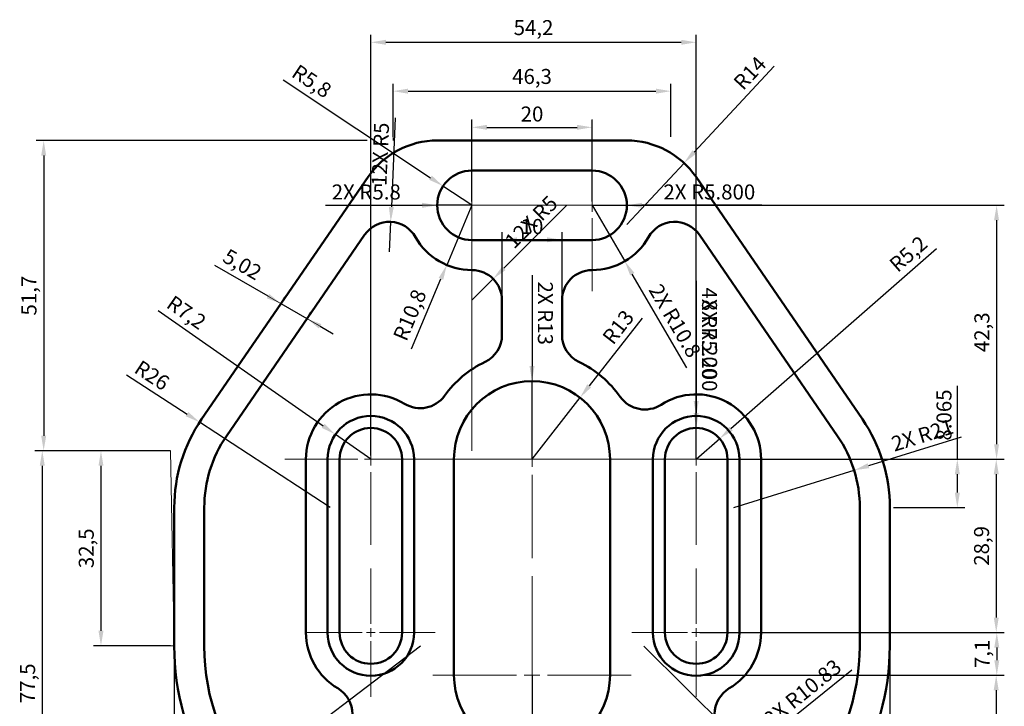
# Model space of a CAD drawing. Units: millimetres. Extents: x 11989 to 12153, y 10398 to 10572.
# Tile 2 of 2: x 11989 to 12153, y 10458 to 10572. Entities that reach past the tile are written whole.
import ezdxf

# ---------------------------------------------------------------- set-up
doc = ezdxf.new("R2010")
doc.units = ezdxf.units.MM
doc.linetypes.add('CENTER', pattern=[50.8, 31.75, -6.35, 6.35, -6.35])
for name, color, linetype, lineweight in [('M-CNTR', 1, 'CENTER', 18), ('M-CONS', 8, 'Continuous', 13), ('M-DIMS', 2, 'Continuous', 25), ('M-OUTL', 7, 'Continuous', 50)]:
    doc.layers.add(name, color=color, linetype=linetype, lineweight=lineweight)
doc.styles.get("Standard").update_dxf_attribs({"font": 'arial.ttf'})
doc.dimstyles.new('ISO-25', dxfattribs={"dimtxt": 2.5, "dimasz": 2.5, "dimexe": 1.25, "dimexo": 0.625, "dimtad": 1, "dimtxsty": 'Standard', "dimcen": 2.5, "dimadec": 0, "dimazin": 0, "dimtfac": 1, "dimtmove": 0, "dimatfit": 3, "dimfxl": 1, "dimarcsym": 0})

# ---------------------------------------------------------------- blocks, each defined once
blk = doc.blocks.new('*U5')
at = {"layer": 'M-CNTR', "color": 0, "transparency": 16777216}
for p, q in [((0, 1.44), (0, 10.7)), ((-10.7, 0), (-1.44, 0)), ((1.44, 0), (10.7, 0)), ((0, -10.7), (0, -1.44))]:
    blk.add_line(p, q, dxfattribs=at)
at = {"layer": 'M-CNTR', "color": 0, "linetype": 'Continuous', "transparency": 16777216}
for p, q in [((-0.72, 0), (0.72, 0)), ((0, -0.72), (0, 0.72))]:
    blk.add_line(p, q, dxfattribs=at)
blk = doc.blocks.new('*U6')
at = {"layer": 'M-CNTR', "color": 0, "transparency": 16777216}
for p, q in [((0, 1.44), (0, 10.7)), ((-10.7, 0), (-1.44, 0)), ((1.44, 0), (10.7, 0)), ((0, -10.7), (0, -1.44))]:
    blk.add_line(p, q, dxfattribs=at)
at = {"layer": 'M-CNTR', "color": 0, "linetype": 'Continuous', "transparency": 16777216}
for p, q in [((-0.72, 0), (0.72, 0)), ((0, -0.72), (0, 0.72))]:
    blk.add_line(p, q, dxfattribs=at)
blk = doc.blocks.new('*U7')
at = {"layer": 'M-CNTR', "color": 0, "transparency": 16777216}
for p, q in [((0, 2.16), (0, 14.3)), ((-14.3, 0), (-2.16, 0)), ((2.16, 0), (14.3, 0)), ((0, -14.3), (0, -2.16))]:
    blk.add_line(p, q, dxfattribs=at)
at = {"layer": 'M-CNTR', "color": 0, "linetype": 'Continuous', "transparency": 16777216}
for p, q in [((-1.08, 0), (1.08, 0)), ((0, -1.08), (0, 1.08))]:
    blk.add_line(p, q, dxfattribs=at)
blk = doc.blocks.new('*U8')
at = {"layer": 'M-CNTR', "color": 0, "transparency": 16777216}
for p, q in [((0, 2.16), (0, 14.3)), ((-14.3, 0), (-2.16, 0)), ((2.16, 0), (14.3, 0)), ((0, -14.3), (0, -2.16))]:
    blk.add_line(p, q, dxfattribs=at)
at = {"layer": 'M-CNTR', "color": 0, "linetype": 'Continuous', "transparency": 16777216}
for p, q in [((-1.08, 0), (1.08, 0)), ((0, -1.08), (0, 1.08))]:
    blk.add_line(p, q, dxfattribs=at)
blk = doc.blocks.new('*U9')
at = {"layer": 'M-CNTR', "color": 0, "transparency": 16777216}
for p, q in [((0, 2.16), (0, 14.3)), ((-14.3, 0), (-2.16, 0)), ((2.16, 0), (14.3, 0)), ((0, -14.3), (0, -2.16))]:
    blk.add_line(p, q, dxfattribs=at)
at = {"layer": 'M-CNTR', "color": 0, "linetype": 'Continuous', "transparency": 16777216}
for p, q in [((-1.08, 0), (1.08, 0)), ((0, -1.08), (0, 1.08))]:
    blk.add_line(p, q, dxfattribs=at)
blk = doc.blocks.new('*U10')
at = {"layer": 'M-CNTR', "color": 0, "transparency": 16777216}
for p, q in [((0, 2.16), (0, 14.3)), ((-14.3, 0), (-2.16, 0)), ((2.16, 0), (14.3, 0)), ((0, -14.3), (0, -2.16))]:
    blk.add_line(p, q, dxfattribs=at)
at = {"layer": 'M-CNTR', "color": 0, "linetype": 'Continuous', "transparency": 16777216}
for p, q in [((-1.08, 0), (1.08, 0)), ((0, -1.08), (0, 1.08))]:
    blk.add_line(p, q, dxfattribs=at)
blk = doc.blocks.new('*U11')
at = {"layer": 'M-CNTR', "color": 0, "transparency": 16777216}
for p, q in [((0, 2.6), (0, 16.5)), ((-16.5, 0), (-2.6, 0)), ((2.6, 0), (16.5, 0)), ((0, -16.5), (0, -2.6))]:
    blk.add_line(p, q, dxfattribs=at)
at = {"layer": 'M-CNTR', "color": 0, "linetype": 'Continuous', "transparency": 16777216}
for p, q in [((-1.3, 0), (1.3, 0)), ((0, -1.3), (0, 1.3))]:
    blk.add_line(p, q, dxfattribs=at)
blk = doc.blocks.new('*U12')
at = {"layer": 'M-CNTR', "color": 0, "transparency": 16777216}
for p, q in [((0, 2.6), (0, 16.5)), ((-16.5, 0), (-2.6, 0)), ((2.6, 0), (16.5, 0)), ((0, -16.5), (0, -2.6))]:
    blk.add_line(p, q, dxfattribs=at)
at = {"layer": 'M-CNTR', "color": 0, "linetype": 'Continuous', "transparency": 16777216}
for p, q in [((-1.3, 0), (1.3, 0)), ((0, -1.3), (0, 1.3))]:
    blk.add_line(p, q, dxfattribs=at)
blk = doc.blocks.new('*D15')
at = {"layer": 'Defpoints', "color": 0, "transparency": 16777216}
for p in [(12014.43, 10479.37), (12133.63, 10479.37), (12133.63, 10399.46)]:
    blk.add_point(p, dxfattribs=at)
at = {"layer": 'M-DIMS', "color": 0, "lineweight": -2, "transparency": 16777216}
for p, q in [((12014.43, 10478.74), (12014.43, 10398.21)), ((12133.63, 10478.74), (12133.63, 10398.21)), ((12016.93, 10399.46), (12131.13, 10399.46))]:
    blk.add_line(p, q, dxfattribs=at)
at = {"layer": 'M-DIMS', "color": 0, "transparency": 16777216}
for points in [[(12016.93, 10399.88), (12016.93, 10399.04), (12014.43, 10399.46)], [(12131.13, 10399.88), (12131.13, 10399.04), (12133.63, 10399.46)]]:
    blk.add_solid(points, dxfattribs=at)
at = {"layer": 'M-DIMS', "color": 0, "transparency": 16777216, "insert": (12074.03, 10401.59), "char_height": 2.5, "attachment_point": 5}
blk.add_mtext('119,2', dxfattribs=at)
blk = doc.blocks.new('*D16')
at = {"layer": 'Defpoints', "color": 0, "transparency": 16777216}
for p in [(12014.43, 10500.37), (12002.23, 10467.87), (12014.43, 10467.87)]:
    blk.add_point(p, dxfattribs=at)
at = {"layer": 'M-DIMS', "color": 0, "lineweight": -2, "transparency": 16777216}
for p, q in [((12013.8, 10500.37), (12000.98, 10500.37)), ((12002.23, 10497.87), (12002.23, 10470.37)), ((12013.8, 10467.87), (12000.98, 10467.87))]:
    blk.add_line(p, q, dxfattribs=at)
at = {"layer": 'M-DIMS', "color": 0, "transparency": 16777216}
for points in [[(12001.81, 10497.87), (12002.64, 10497.87), (12002.23, 10500.37)], [(12001.81, 10470.37), (12002.64, 10470.37), (12002.23, 10467.87)]]:
    blk.add_solid(points, dxfattribs=at)
at = {"layer": 'M-DIMS', "color": 0, "transparency": 16777216, "insert": (12000.1, 10484.12), "char_height": 2.5, "attachment_point": 5, "rotation": 90}
blk.add_mtext('32,5', dxfattribs=at)
blk = doc.blocks.new('*D17')
at = {"layer": 'Defpoints', "color": 0, "transparency": 16777216}
for p in [(12084.03, 10554.26), (12064.03, 10541.27), (12084.03, 10541.27)]:
    blk.add_point(p, dxfattribs=at)
at = {"layer": 'M-DIMS', "color": 0, "lineweight": -2, "transparency": 16777216}
for p, q in [((12064.03, 10541.9), (12064.03, 10555.51)), ((12084.03, 10541.9), (12084.03, 10555.51)), ((12066.53, 10554.26), (12081.53, 10554.26))]:
    blk.add_line(p, q, dxfattribs=at)
at = {"layer": 'M-DIMS', "color": 0, "transparency": 16777216}
for points in [[(12066.53, 10554.68), (12066.53, 10553.85), (12064.03, 10554.26)], [(12081.53, 10554.68), (12081.53, 10553.85), (12084.03, 10554.26)]]:
    blk.add_solid(points, dxfattribs=at)
at = {"layer": 'M-DIMS', "color": 0, "transparency": 16777216, "insert": (12074.03, 10556.16), "char_height": 2.5, "attachment_point": 5}
blk.add_mtext('20', dxfattribs=at)
blk = doc.blocks.new('*D18')
at = {"layer": 'Defpoints', "color": 0, "transparency": 16777216}
for p in [(12097.18, 10560.29), (12050.88, 10552.07), (12097.18, 10552.07)]:
    blk.add_point(p, dxfattribs=at)
at = {"layer": 'M-DIMS', "color": 0, "lineweight": -2, "transparency": 16777216}
for p, q in [((12050.88, 10552.7), (12050.88, 10561.54)), ((12097.18, 10552.7), (12097.18, 10561.54)), ((12053.38, 10560.29), (12094.68, 10560.29))]:
    blk.add_line(p, q, dxfattribs=at)
at = {"layer": 'M-DIMS', "color": 0, "transparency": 16777216}
for points in [[(12053.38, 10560.71), (12053.38, 10559.87), (12050.88, 10560.29)], [(12094.68, 10560.71), (12094.68, 10559.87), (12097.18, 10560.29)]]:
    blk.add_solid(points, dxfattribs=at)
at = {"layer": 'M-DIMS', "color": 0, "transparency": 16777216, "insert": (12074.03, 10562.42), "char_height": 2.5, "attachment_point": 5}
blk.add_mtext('46,3', dxfattribs=at)
blk = doc.blocks.new('*D19')
at = {"layer": 'Defpoints', "color": 0, "transparency": 16777216}
for p in [(12101.38, 10568.43), (12047.18, 10498.97), (12101.38, 10498.97)]:
    blk.add_point(p, dxfattribs=at)
at = {"layer": 'M-DIMS', "color": 0, "lineweight": -2, "transparency": 16777216}
for p, q in [((12047.18, 10499.6), (12047.18, 10569.68)), ((12101.38, 10499.6), (12101.38, 10569.68)), ((12049.68, 10568.43), (12098.88, 10568.43))]:
    blk.add_line(p, q, dxfattribs=at)
at = {"layer": 'M-DIMS', "color": 0, "transparency": 16777216}
for points in [[(12049.68, 10568.85), (12049.68, 10568.02), (12047.18, 10568.43)], [(12098.88, 10568.85), (12098.88, 10568.02), (12101.38, 10568.43)]]:
    blk.add_solid(points, dxfattribs=at)
at = {"layer": 'M-DIMS', "color": 0, "transparency": 16777216, "insert": (12074.28, 10570.56), "char_height": 2.5, "attachment_point": 5}
blk.add_mtext('54,2', dxfattribs=at)
blk = doc.blocks.new('*D20')
at = {"layer": 'Defpoints', "color": 0, "transparency": 16777216}
for p in [(12099.35, 10548.32), (12089.81, 10538.07)]:
    blk.add_point(p, dxfattribs=at)
at = {"layer": 'M-DIMS', "color": 0, "lineweight": -2, "transparency": 16777216}
for p, q in [((12114.38, 10564.45), (12101.06, 10550.15)), ((12089.81, 10538.07), (12099.35, 10548.32))]:
    blk.add_line(p, q, dxfattribs=at)
at = {"layer": 'M-DIMS', "color": 0, "transparency": 16777216}
blk.add_solid([(12100.75, 10550.43), (12101.36, 10549.86), (12099.35, 10548.32)], dxfattribs=at)
at = {"layer": 'M-DIMS', "color": 0, "transparency": 16777216, "insert": (12110.55, 10563.09), "char_height": 2.5, "attachment_point": 5, "rotation": 47.0295}
blk.add_mtext('R14', dxfattribs=at)
blk = doc.blocks.new('*D21')
at = {"layer": 'Defpoints', "color": 0, "transparency": 16777216}
for p in [(12059.2, 10544.48), (12064.03, 10541.27)]:
    blk.add_point(p, dxfattribs=at)
at = {"layer": 'M-DIMS', "color": 0, "lineweight": -2, "transparency": 16777216}
for p, q in [((12032.57, 10562.19), (12057.12, 10545.87)), ((12064.03, 10541.27), (12059.2, 10544.48))]:
    blk.add_line(p, q, dxfattribs=at)
at = {"layer": 'M-DIMS', "color": 0, "transparency": 16777216}
blk.add_solid([(12057.35, 10546.21), (12056.89, 10545.52), (12059.2, 10544.48)], dxfattribs=at)
at = {"layer": 'M-DIMS', "color": 0, "transparency": 16777216, "insert": (12037.16, 10561.69), "char_height": 2.5, "attachment_point": 5, "rotation": 326.3843}
blk.add_mtext('R5,8', dxfattribs=at)
blk = doc.blocks.new('*D22')
at = {"layer": 'Defpoints', "color": 0, "transparency": 16777216}
for p in [(12041.28, 10503.1), (12047.18, 10498.97)]:
    blk.add_point(p, dxfattribs=at)
at = {"layer": 'M-DIMS', "color": 0, "lineweight": -2, "transparency": 16777216}
for p, q in [((12011.73, 10523.74), (12039.23, 10504.53)), ((12047.18, 10498.97), (12041.28, 10503.1))]:
    blk.add_line(p, q, dxfattribs=at)
at = {"layer": 'M-DIMS', "color": 0, "transparency": 16777216}
blk.add_solid([(12039.47, 10504.87), (12038.99, 10504.19), (12041.28, 10503.1)], dxfattribs=at)
at = {"layer": 'M-DIMS', "color": 0, "transparency": 16777216, "insert": (12016.29, 10523.15), "char_height": 2.5, "attachment_point": 5, "rotation": 325.0597}
blk.add_mtext('R7,2', dxfattribs=at)
blk = doc.blocks.new('*D23')
at = {"layer": 'Defpoints', "color": 0, "transparency": 16777216}
for p in [(12018.66, 10505.12), (12040.43, 10490.91)]:
    blk.add_point(p, dxfattribs=at)
at = {"layer": 'M-DIMS', "color": 0, "lineweight": -2, "transparency": 16777216}
for p, q in [((12006.5, 10513.05), (12016.56, 10506.48)), ((12040.43, 10490.91), (12018.66, 10505.12))]:
    blk.add_line(p, q, dxfattribs=at)
at = {"layer": 'M-DIMS', "color": 0, "transparency": 16777216}
blk.add_solid([(12016.79, 10506.83), (12016.33, 10506.13), (12018.66, 10505.12)], dxfattribs=at)
at = {"layer": 'M-DIMS', "color": 0, "transparency": 16777216, "insert": (12010.56, 10512.67), "char_height": 2.5, "attachment_point": 5, "rotation": 326.8734}
blk.add_mtext('R26', dxfattribs=at)
blk = doc.blocks.new('*D24')
at = {"layer": 'Defpoints', "color": 0, "transparency": 16777216}
for p in [(12032.22, 10524.88), (12032.22, 10524.88), (12036.56, 10522.37)]:
    blk.add_point(p, dxfattribs=at)
at = {"layer": 'M-DIMS', "color": 0, "lineweight": -2, "transparency": 16777216}
for p, q in [((12030.05, 10526.13), (12021.2, 10531.24)), ((12032.53, 10525.42), (12032.84, 10525.96)), ((12036.56, 10522.37), (12032.22, 10524.88)), ((12036.87, 10522.92), (12037.18, 10523.46)), ((12038.72, 10521.12), (12040.89, 10519.87))]:
    blk.add_line(p, q, dxfattribs=at)
at = {"layer": 'M-DIMS', "color": 0, "transparency": 16777216}
for points in [[(12030.26, 10526.49), (12029.84, 10525.77), (12032.22, 10524.88)], [(12038.93, 10521.49), (12038.52, 10520.76), (12036.56, 10522.37)]]:
    blk.add_solid(points, dxfattribs=at)
at = {"layer": 'M-DIMS', "color": 0, "transparency": 16777216, "insert": (12025.61, 10531.15), "char_height": 2.5, "attachment_point": 5, "rotation": 330}
blk.add_mtext('5,02', dxfattribs=at)
blk = doc.blocks.new('*D25')
at = {"layer": 'Defpoints', "color": 0, "transparency": 16777216}
for p in [(12064.03, 10541.27), (12059.83, 10531.32)]:
    blk.add_point(p, dxfattribs=at)
at = {"layer": 'M-DIMS', "color": 0, "lineweight": -2, "transparency": 16777216}
for p, q in [((12064.03, 10541.27), (12059.83, 10531.32)), ((12053.95, 10517.37), (12058.86, 10529.02))]:
    blk.add_line(p, q, dxfattribs=at)
at = {"layer": 'M-DIMS', "color": 0, "transparency": 16777216}
blk.add_solid([(12058.48, 10529.18), (12059.24, 10528.86), (12059.83, 10531.32)], dxfattribs=at)
at = {"layer": 'M-DIMS', "color": 0, "transparency": 16777216, "insert": (12053.96, 10522.87), "char_height": 2.5, "attachment_point": 5, "rotation": 67.132}
blk.add_mtext('R10,8', dxfattribs=at)
blk = doc.blocks.new('*D26')
at = {"layer": 'Defpoints', "color": 0, "transparency": 16777216}
for p in [(12082.03, 10509.22), (12074.03, 10498.97)]:
    blk.add_point(p, dxfattribs=at)
at = {"layer": 'M-DIMS', "color": 0, "lineweight": -2, "transparency": 16777216}
for p, q in [((12092.36, 10522.46), (12083.56, 10511.19)), ((12074.03, 10498.97), (12082.03, 10509.22))]:
    blk.add_line(p, q, dxfattribs=at)
at = {"layer": 'M-DIMS', "color": 0, "transparency": 16777216}
blk.add_solid([(12083.24, 10511.45), (12083.89, 10510.94), (12082.03, 10509.22)], dxfattribs=at)
at = {"layer": 'M-DIMS', "color": 0, "transparency": 16777216, "insert": (12088.64, 10520.78), "char_height": 2.5, "attachment_point": 5, "rotation": 52.0351}
blk.add_mtext('R13', dxfattribs=at)
blk = doc.blocks.new('*D30')
at = {"layer": 'Defpoints', "color": 0, "transparency": 16777216}
for p in [(12055.43, 10467.83), (12022.79, 10443.01)]:
    blk.add_point(p, dxfattribs=at)
at = {"layer": 'M-DIMS', "color": 0, "lineweight": -2, "transparency": 16777216}
for p, q in [((12055.43, 10467.83), (12022.79, 10443.01)), ((12001.8, 10427.05), (12020.8, 10441.5))]:
    blk.add_line(p, q, dxfattribs=at)
at = {"layer": 'M-DIMS', "color": 0, "transparency": 16777216}
blk.add_solid([(12020.55, 10441.83), (12021.06, 10441.17), (12022.79, 10443.01)], dxfattribs=at)
at = {"layer": 'M-DIMS', "color": 0, "transparency": 16777216, "insert": (12003.35, 10430.59), "char_height": 2.5, "attachment_point": 5, "rotation": 37.2506}
blk.add_mtext('R41', dxfattribs=at)
blk = doc.blocks.new('*D32')
at = {"layer": 'Defpoints', "color": 0, "transparency": 16777216}
for p in [(12047.18, 10552.07), (11992.68, 10500.37), (12013.8, 10500.37)]:
    blk.add_point(p, dxfattribs=at)
at = {"layer": 'M-DIMS', "color": 0, "lineweight": -2, "transparency": 16777216}
for p, q in [((12046.55, 10552.07), (11991.43, 10552.07)), ((11992.68, 10549.57), (11992.68, 10502.87)), ((12013.18, 10500.37), (11991.43, 10500.37))]:
    blk.add_line(p, q, dxfattribs=at)
at = {"layer": 'M-DIMS', "color": 0, "transparency": 16777216}
for points in [[(11992.27, 10549.57), (11993.1, 10549.57), (11992.68, 10552.07)], [(11992.27, 10502.87), (11993.1, 10502.87), (11992.68, 10500.37)]]:
    blk.add_solid(points, dxfattribs=at)
at = {"layer": 'M-DIMS', "color": 0, "transparency": 16777216, "insert": (11990.56, 10526.22), "char_height": 2.5, "attachment_point": 5, "rotation": 90}
blk.add_mtext('51,7', dxfattribs=at)
blk = doc.blocks.new('*D33')
at = {"layer": 'Defpoints', "color": 0, "transparency": 16777216}
for p in [(11992.68, 10500.37), (11992.45, 10422.87), (12049.1, 10422.87)]:
    blk.add_point(p, dxfattribs=at)
at = {"layer": 'M-DIMS', "color": 0, "lineweight": -2, "transparency": 16777216}
for p, q in [((11992.06, 10500.37), (11991.2, 10500.37)), ((11992.45, 10497.87), (11992.45, 10425.37)), ((12048.47, 10422.87), (11991.2, 10422.87))]:
    blk.add_line(p, q, dxfattribs=at)
at = {"layer": 'M-DIMS', "color": 0, "transparency": 16777216}
for points in [[(11992.03, 10497.87), (11992.87, 10497.87), (11992.45, 10500.37)], [(11992.03, 10425.37), (11992.87, 10425.37), (11992.45, 10422.87)]]:
    blk.add_solid(points, dxfattribs=at)
at = {"layer": 'M-DIMS', "color": 0, "transparency": 16777216, "insert": (11990.33, 10461.62), "char_height": 2.5, "attachment_point": 5, "rotation": 90}
blk.add_mtext('77,5', dxfattribs=at)
blk = doc.blocks.new('*D34')
at = {"layer": 'Defpoints', "color": 0, "transparency": 16777216}
for p in [(12084.03, 10541.27), (12101.38, 10498.97), (12151.42, 10498.97)]:
    blk.add_point(p, dxfattribs=at)
at = {"layer": 'M-DIMS', "color": 0, "lineweight": -2, "transparency": 16777216}
for p, q in [((12084.65, 10541.27), (12152.67, 10541.27)), ((12151.42, 10538.77), (12151.42, 10501.47)), ((12102, 10498.97), (12152.67, 10498.97))]:
    blk.add_line(p, q, dxfattribs=at)
at = {"layer": 'M-DIMS', "color": 0, "transparency": 16777216}
for points in [[(12151, 10538.77), (12151.83, 10538.77), (12151.42, 10541.27)], [(12151, 10501.47), (12151.83, 10501.47), (12151.42, 10498.97)]]:
    blk.add_solid(points, dxfattribs=at)
at = {"layer": 'M-DIMS', "color": 0, "transparency": 16777216, "insert": (12149.29, 10520.12), "char_height": 2.5, "attachment_point": 5, "rotation": 90}
blk.add_mtext('42,3', dxfattribs=at)
blk = doc.blocks.new('*D35')
at = {"layer": 'Defpoints', "color": 0, "transparency": 16777216}
for p in [(12101.38, 10498.97), (12101.38, 10470.07), (12151.36, 10470.07)]:
    blk.add_point(p, dxfattribs=at)
at = {"layer": 'M-DIMS', "color": 0, "lineweight": -2, "transparency": 16777216}
for p, q in [((12102, 10498.97), (12152.61, 10498.97)), ((12151.36, 10496.47), (12151.36, 10472.57)), ((12102, 10470.07), (12152.61, 10470.07))]:
    blk.add_line(p, q, dxfattribs=at)
at = {"layer": 'M-DIMS', "color": 0, "transparency": 16777216}
for points in [[(12150.95, 10496.47), (12151.78, 10496.47), (12151.36, 10498.97)], [(12150.95, 10472.57), (12151.78, 10472.57), (12151.36, 10470.07)]]:
    blk.add_solid(points, dxfattribs=at)
at = {"layer": 'M-DIMS', "color": 0, "transparency": 16777216, "insert": (12149.24, 10484.52), "char_height": 2.5, "attachment_point": 5, "rotation": 90}
blk.add_mtext('28,9', dxfattribs=at)
blk = doc.blocks.new('*D36')
at = {"layer": 'Defpoints', "color": 0, "transparency": 16777216}
for p in [(12101.38, 10470.07), (12101.38, 10462.97), (12151.45, 10462.97)]:
    blk.add_point(p, dxfattribs=at)
at = {"layer": 'M-DIMS', "color": 0, "lineweight": -2, "transparency": 16777216}
for p, q in [((12102, 10470.07), (12152.7, 10470.07)), ((12151.45, 10467.57), (12151.45, 10465.47)), ((12102, 10462.97), (12152.7, 10462.97))]:
    blk.add_line(p, q, dxfattribs=at)
at = {"layer": 'M-DIMS', "color": 0, "transparency": 16777216}
for points in [[(12151.04, 10467.57), (12151.87, 10467.57), (12151.45, 10470.07)], [(12151.04, 10465.47), (12151.87, 10465.47), (12151.45, 10462.97)]]:
    blk.add_solid(points, dxfattribs=at)
at = {"layer": 'M-DIMS', "color": 0, "transparency": 16777216, "insert": (12149.33, 10466.52), "char_height": 2.5, "attachment_point": 5, "rotation": 90}
blk.add_mtext('7,1', dxfattribs=at)
blk = doc.blocks.new('*D37')
at = {"layer": 'Defpoints', "color": 0, "transparency": 16777216}
for p in [(12102.04, 10462.97), (12101.38, 10442.87), (12151.35, 10442.87)]:
    blk.add_point(p, dxfattribs=at)
at = {"layer": 'M-DIMS', "color": 0, "lineweight": -2, "transparency": 16777216}
for p, q in [((12102.66, 10462.97), (12152.6, 10462.97)), ((12151.35, 10460.47), (12151.35, 10445.37)), ((12102, 10442.87), (12152.6, 10442.87))]:
    blk.add_line(p, q, dxfattribs=at)
at = {"layer": 'M-DIMS', "color": 0, "transparency": 16777216}
for points in [[(12150.94, 10460.47), (12151.77, 10460.47), (12151.35, 10462.97)], [(12150.94, 10445.37), (12151.77, 10445.37), (12151.35, 10442.87)]]:
    blk.add_solid(points, dxfattribs=at)
at = {"layer": 'M-DIMS', "color": 0, "transparency": 16777216, "insert": (12149.23, 10452.92), "char_height": 2.5, "attachment_point": 5, "rotation": 90}
blk.add_mtext('20,1', dxfattribs=at)
blk = doc.blocks.new('*D38')
at = {"layer": 'Defpoints', "color": 0, "transparency": 16777216}
for p in [(12105.29, 10502.4), (12101.38, 10498.97)]:
    blk.add_point(p, dxfattribs=at)
at = {"layer": 'M-DIMS', "color": 0, "lineweight": -2, "transparency": 16777216}
for p, q in [((12141.4, 10534.03), (12107.17, 10504.05)), ((12101.38, 10498.97), (12105.29, 10502.4))]:
    blk.add_line(p, q, dxfattribs=at)
at = {"layer": 'M-DIMS', "color": 0, "transparency": 16777216}
blk.add_solid([(12106.9, 10504.36), (12107.45, 10503.73), (12105.29, 10502.4)], dxfattribs=at)
at = {"layer": 'M-DIMS', "color": 0, "transparency": 16777216, "insert": (12136.93, 10532.94), "char_height": 2.5, "attachment_point": 5, "rotation": 41.2173}
blk.add_mtext('R5,2', dxfattribs=at)
blk = doc.blocks.new('*D39')
at = {"layer": 'Defpoints', "color": 0, "transparency": 16777216}
for p in [(12079.03, 10535.52), (12069.03, 10525.47), (12079.03, 10525.47)]:
    blk.add_point(p, dxfattribs=at)
at = {"layer": 'M-DIMS', "color": 0, "lineweight": -2, "transparency": 16777216}
for p, q in [((12069.03, 10526.1), (12069.03, 10536.77)), ((12079.03, 10526.1), (12079.03, 10536.77)), ((12071.53, 10535.52), (12076.53, 10535.52))]:
    blk.add_line(p, q, dxfattribs=at)
at = {"layer": 'M-DIMS', "color": 0, "transparency": 16777216}
for points in [[(12071.53, 10535.94), (12071.53, 10535.11), (12069.03, 10535.52)], [(12076.53, 10535.94), (12076.53, 10535.11), (12079.03, 10535.52)]]:
    blk.add_solid(points, dxfattribs=at)
at = {"layer": 'M-DIMS', "color": 0, "transparency": 16777216, "insert": (12074.03, 10537.42), "char_height": 2.5, "attachment_point": 5}
blk.add_mtext('10', dxfattribs=at)
blk = doc.blocks.new('*D40')
at = {"layer": 'Defpoints', "color": 0, "transparency": 16777216}
for p in [(12092.63, 10467.83), (12121.79, 10439.01)]:
    blk.add_point(p, dxfattribs=at)
at = {"layer": 'M-DIMS', "color": 0, "lineweight": -2, "transparency": 16777216}
for p, q in [((12092.63, 10467.83), (12121.79, 10439.01)), ((12143.61, 10417.44), (12123.57, 10437.25))]:
    blk.add_line(p, q, dxfattribs=at)
at = {"layer": 'M-DIMS', "color": 0, "transparency": 16777216}
blk.add_solid([(12123.86, 10437.55), (12123.27, 10436.96), (12121.79, 10439.01)], dxfattribs=at)
at = {"layer": 'M-DIMS', "color": 0, "transparency": 16777216, "insert": (12140.61, 10423.06), "char_height": 2.5, "attachment_point": 5, "rotation": 315.3343}
blk.add_mtext('2X R41', dxfattribs=at)
blk = doc.blocks.new('*D41')
at = {"layer": 'Defpoints', "color": 0, "transparency": 16777216}
for p in [(12127.69, 10497.13), (12107.63, 10490.91)]:
    blk.add_point(p, dxfattribs=at)
at = {"layer": 'M-DIMS', "color": 0, "lineweight": -2, "transparency": 16777216}
for p, q in [((12145.53, 10502.66), (12130.07, 10497.87)), ((12107.63, 10490.91), (12127.69, 10497.13))]:
    blk.add_line(p, q, dxfattribs=at)
at = {"layer": 'M-DIMS', "color": 0, "transparency": 16777216}
blk.add_solid([(12129.95, 10498.27), (12130.2, 10497.47), (12127.69, 10497.13)], dxfattribs=at)
at = {"layer": 'M-DIMS', "color": 0, "transparency": 16777216, "insert": (12139.16, 10502.66), "char_height": 2.5, "attachment_point": 5, "rotation": 17.2339}
blk.add_mtext('2X R21', dxfattribs=at)
blk = doc.blocks.new('*D42')
at = {"layer": 'Defpoints', "color": 0, "transparency": 16777216}
for p in [(12074.03, 10511.97), (12074.03, 10498.97)]:
    blk.add_point(p, dxfattribs=at)
at = {"layer": 'M-DIMS', "color": 0, "lineweight": -2, "transparency": 16777216}
for p, q in [((12074.03, 10529.61), (12074.03, 10514.47)), ((12074.03, 10498.97), (12074.03, 10511.97))]:
    blk.add_line(p, q, dxfattribs=at)
at = {"layer": 'M-DIMS', "color": 0, "transparency": 16777216}
blk.add_solid([(12074.45, 10514.47), (12073.61, 10514.47), (12074.03, 10511.97)], dxfattribs=at)
at = {"layer": 'M-DIMS', "color": 0, "transparency": 16777216, "insert": (12075.93, 10523.29), "char_height": 2.5, "attachment_point": 5, "rotation": 270.002}
blk.add_mtext('2X R13', dxfattribs=at)
blk = doc.blocks.new('*D43')
at = {"layer": 'Defpoints', "color": 0, "transparency": 16777216}
for p in [(12109.8, 10449.68), (12101.38, 10442.87)]:
    blk.add_point(p, dxfattribs=at)
at = {"layer": 'M-DIMS', "color": 0, "lineweight": -2, "transparency": 16777216}
for p, q in [((12127.29, 10463.82), (12111.74, 10451.25)), ((12101.38, 10442.87), (12109.8, 10449.68))]:
    blk.add_line(p, q, dxfattribs=at)
at = {"layer": 'M-DIMS', "color": 0, "transparency": 16777216}
blk.add_solid([(12111.48, 10451.58), (12112.01, 10450.93), (12109.8, 10449.68)], dxfattribs=at)
at = {"layer": 'M-DIMS', "color": 0, "transparency": 16777216, "insert": (12119.29, 10459.8), "char_height": 2.5, "attachment_point": 5, "rotation": 38.9595}
blk.add_mtext('2X R10.83', dxfattribs=at)
blk = doc.blocks.new('*D44')
at = {"layer": 'Defpoints', "color": 0, "transparency": 16777216}
for p in [(12058.23, 10541.27), (12064.03, 10541.27)]:
    blk.add_point(p, dxfattribs=at)
at = {"layer": 'M-DIMS', "color": 0, "lineweight": -2, "transparency": 16777216}
for p, q in [((12039.62, 10541.27), (12055.73, 10541.27)), ((12064.03, 10541.27), (12058.23, 10541.27))]:
    blk.add_line(p, q, dxfattribs=at)
at = {"layer": 'M-DIMS', "color": 0, "transparency": 16777216}
blk.add_solid([(12055.73, 10541.69), (12055.73, 10540.86), (12058.23, 10541.27)], dxfattribs=at)
at = {"layer": 'M-DIMS', "color": 0, "transparency": 16777216, "insert": (12046.42, 10543.17), "char_height": 2.5, "attachment_point": 5, "rotation": 0.002}
blk.add_mtext('2X R5.8', dxfattribs=at)
blk = doc.blocks.new('*D45')
at = {"layer": 'Defpoints', "color": 0, "transparency": 16777216}
for p in [(12067.56, 10529.01), (12064.03, 10525.47)]:
    blk.add_point(p, dxfattribs=at)
at = {"layer": 'M-DIMS', "color": 0, "lineweight": -2, "transparency": 16777216}
for p, q in [((12079.85, 10541.3), (12069.33, 10530.78)), ((12064.03, 10525.47), (12067.56, 10529.01))]:
    blk.add_line(p, q, dxfattribs=at)
at = {"layer": 'M-DIMS', "color": 0, "transparency": 16777216}
blk.add_solid([(12069.04, 10531.07), (12069.63, 10530.48), (12067.56, 10529.01)], dxfattribs=at)
at = {"layer": 'M-DIMS', "color": 0, "transparency": 16777216, "insert": (12074.13, 10538.26), "char_height": 2.5, "attachment_point": 5, "rotation": 45.002}
blk.add_mtext('12X R5', dxfattribs=at)
blk = doc.blocks.new('*D46')
at = {"layer": 'Defpoints', "color": 0, "transparency": 16777216}
for p in [(12101.38, 10498.97), (12144.88, 10498.97), (12133.63, 10490.91)]:
    blk.add_point(p, dxfattribs=at)
at = {"layer": 'M-DIMS', "color": 0, "lineweight": -2, "transparency": 16777216}
for p, q in [((12144.88, 10498.97), (12144.88, 10511.18)), ((12102, 10498.97), (12146.13, 10498.97)), ((12144.88, 10493.41), (12144.88, 10496.47)), ((12134.25, 10490.91), (12146.13, 10490.91))]:
    blk.add_line(p, q, dxfattribs=at)
at = {"layer": 'M-DIMS', "color": 0, "transparency": 16777216}
for points in [[(12144.46, 10496.47), (12145.3, 10496.47), (12144.88, 10498.97)], [(12144.46, 10493.41), (12145.3, 10493.41), (12144.88, 10490.91)]]:
    blk.add_solid(points, dxfattribs=at)
at = {"layer": 'M-DIMS', "color": 0, "transparency": 16777216, "insert": (12142.98, 10506.33), "char_height": 2.5, "attachment_point": 5, "rotation": 90}
blk.add_mtext('8.065', dxfattribs=at)
blk = doc.blocks.new('*D47')
at = {"layer": 'Defpoints', "color": 0, "transparency": 16777216}
for p in [(12074.03, 10462.97), (12074.03, 10449.97)]:
    blk.add_point(p, dxfattribs=at)
at = {"layer": 'M-DIMS', "color": 0, "lineweight": -2, "transparency": 16777216}
for p, q in [((12074.03, 10462.97), (12074.03, 10449.97)), ((12074.03, 10432.33), (12074.03, 10447.47))]:
    blk.add_line(p, q, dxfattribs=at)
at = {"layer": 'M-DIMS', "color": 0, "transparency": 16777216}
blk.add_solid([(12073.61, 10447.47), (12074.45, 10447.47), (12074.03, 10449.97)], dxfattribs=at)
at = {"layer": 'M-DIMS', "color": 0, "transparency": 16777216, "insert": (12072.13, 10438.65), "char_height": 2.5, "attachment_point": 5, "rotation": 89.998}
blk.add_mtext('2X R13', dxfattribs=at)
blk = doc.blocks.new('*D48')
at = {"layer": 'Defpoints', "color": 0, "transparency": 16777216}
for p in [(12050.49, 10538.51), (12050.27, 10533.51)]:
    blk.add_point(p, dxfattribs=at)
at = {"layer": 'M-DIMS', "color": 0, "lineweight": -2, "transparency": 16777216}
for p, q in [((12051.25, 10555.87), (12050.6, 10541)), ((12050.27, 10533.51), (12050.49, 10538.51))]:
    blk.add_line(p, q, dxfattribs=at)
at = {"layer": 'M-DIMS', "color": 0, "transparency": 16777216}
blk.add_solid([(12050.18, 10541.02), (12051.01, 10540.99), (12050.49, 10538.51)], dxfattribs=at)
at = {"layer": 'M-DIMS', "color": 0, "transparency": 16777216, "insert": (12049.08, 10549.77), "char_height": 2.5, "attachment_point": 5, "rotation": 87.4817}
blk.add_mtext('12X R5', dxfattribs=at)
blk = doc.blocks.new('*D50')
at = {"layer": 'Defpoints', "color": 0, "transparency": 16777216}
for p in [(12084.03, 10541.27), (12089.48, 10531.95)]:
    blk.add_point(p, dxfattribs=at)
at = {"layer": 'M-DIMS', "color": 0, "lineweight": -2, "transparency": 16777216}
for p, q in [((12084.03, 10541.27), (12089.48, 10531.95)), ((12099.84, 10514.2), (12090.74, 10529.79))]:
    blk.add_line(p, q, dxfattribs=at)
at = {"layer": 'M-DIMS', "color": 0, "transparency": 16777216}
blk.add_solid([(12091.1, 10530), (12090.38, 10529.58), (12089.48, 10531.95)], dxfattribs=at)
at = {"layer": 'M-DIMS', "color": 0, "transparency": 16777216, "insert": (12097.56, 10521.87), "char_height": 2.5, "attachment_point": 5, "rotation": 300.2897}
blk.add_mtext('2X R10.8', dxfattribs=at)
blk = doc.blocks.new('*D51')
at = {"layer": 'Defpoints', "color": 0, "transparency": 16777216}
for p in [(12101.38, 10506.17), (12101.38, 10498.97)]:
    blk.add_point(p, dxfattribs=at)
at = {"layer": 'M-DIMS', "color": 0, "lineweight": -2, "transparency": 16777216}
for p, q in [((12101.38, 10528.71), (12101.38, 10508.67)), ((12101.38, 10498.97), (12101.38, 10506.17))]:
    blk.add_line(p, q, dxfattribs=at)
at = {"layer": 'M-DIMS', "color": 0, "transparency": 16777216}
blk.add_solid([(12101.8, 10508.67), (12100.96, 10508.67), (12101.38, 10506.17)], dxfattribs=at)
at = {"layer": 'M-DIMS', "color": 0, "transparency": 16777216, "insert": (12103.28, 10519.94), "char_height": 2.5, "attachment_point": 5, "rotation": 270.0036}
blk.add_mtext('4X R7.200', dxfattribs=at)
blk = doc.blocks.new('*D52')
at = {"layer": 'Defpoints', "color": 0, "transparency": 16777216}
for p in [(12084.03, 10541.27), (12089.83, 10541.27)]:
    blk.add_point(p, dxfattribs=at)
at = {"layer": 'M-DIMS', "color": 0, "lineweight": -2, "transparency": 16777216}
for p, q in [((12084.03, 10541.27), (12089.83, 10541.27)), ((12112.31, 10541.27), (12092.33, 10541.27))]:
    blk.add_line(p, q, dxfattribs=at)
at = {"layer": 'M-DIMS', "color": 0, "transparency": 16777216}
blk.add_solid([(12092.33, 10541.69), (12092.33, 10540.86), (12089.83, 10541.27)], dxfattribs=at)
at = {"layer": 'M-DIMS', "color": 0, "transparency": 16777216, "insert": (12103.57, 10543.17), "char_height": 2.5, "attachment_point": 5, "rotation": 359.998}
blk.add_mtext('2X R5.800', dxfattribs=at)
blk = doc.blocks.new('*D53')
at = {"layer": 'Defpoints', "color": 0, "transparency": 16777216}
for p in [(12101.38, 10504.17), (12101.38, 10498.97)]:
    blk.add_point(p, dxfattribs=at)
at = {"layer": 'M-DIMS', "color": 0, "lineweight": -2, "transparency": 16777216}
for p, q in [((12101.38, 10526.62), (12101.38, 10506.67)), ((12101.38, 10498.97), (12101.38, 10504.17))]:
    blk.add_line(p, q, dxfattribs=at)
at = {"layer": 'M-DIMS', "color": 0, "transparency": 16777216}
blk.add_solid([(12101.8, 10506.67), (12100.96, 10506.67), (12101.38, 10504.17)], dxfattribs=at)
at = {"layer": 'M-DIMS', "color": 0, "transparency": 16777216, "insert": (12103.28, 10517.9), "char_height": 2.5, "attachment_point": 5, "rotation": 270.005}
blk.add_mtext('8X R5.200', dxfattribs=at)

msp = doc.modelspace()

# ---------------------------------------------------------------- linework, layer by layer
at = {"layer": 'M-CONS'}
for p, q in [((12050.8795, 10552.0722), (12050.8795, 10555.1058)), ((12074.0295, 10552.0722), (12058.2503, 10552.0722)), ((12064.0295, 10552.0722), (12084.0295, 10552.0722)), ((12064.0295, 10552.0722), (12064.0295, 10500.3722)), ((12064.0295, 10541.2722), (12084.0295, 10541.2722)), ((12064.0295, 10530.4722), (12064.0295, 10530.4722)), ((12028.7099, 10526.9057), (12039.4099, 10520.7281)), ((12013.8045, 10500.3722), (12014.4295, 10467.8321)), ((12101.3795, 10498.9722), (12047.1795, 10498.9722)), ((12101.3795, 10498.9722), (12047.1795, 10498.9722)), ((12074.0295, 10498.9722), (12101.3795, 10498.9722)), ((12074.0295, 10498.9722), (12101.3795, 10498.9722)), ((12101.3795, 10498.9722), (12125.9765, 10498.9722)), ((12125.9765, 10498.9722), (12127.019, 10498.9722)), ((12074.0295, 10470.0722), (12074.0295, 10462.9722)), ((12101.3795, 10470.0722), (12125.9765, 10470.0722)), ((12101.3795, 10470.0722), (12128.6295, 10470.0722)), ((12014.4295, 10467.8722), (12012.7243, 10467.8722))]:
    msp.add_line(p, q, dxfattribs=at)
at = {"layer": 'M-OUTL'}
for p, q in [((12058.2503, 10552.0722), (12089.8086, 10552.0722)), ((12064.0295, 10547.0722), (12084.0295, 10547.0722)), ((12064.0295, 10535.4722), (12084.0295, 10535.4722)), ((12069.0295, 10519.6845), (12069.0295, 10525.4722)), ((12079.0295, 10519.6845), (12079.0295, 10525.4722)), ((12036.3795, 10498.9722), (12036.3795, 10470.0722)), ((12039.9795, 10498.9722), (12039.9795, 10470.0722)), ((12041.9795, 10498.9722), (12041.9795, 10470.0722)), ((12052.3795, 10498.9722), (12052.3795, 10470.0722)), ((12054.3795, 10498.9722), (12054.3795, 10470.0722)), ((12061.0295, 10498.9722), (12061.0295, 10462.9722)), ((12087.0295, 10498.9722), (12087.0295, 10462.9722)), ((12094.1795, 10498.9722), (12094.1795, 10470.0722)), ((12096.1795, 10498.9722), (12096.1795, 10470.0722)), ((12106.5795, 10498.9722), (12106.5795, 10470.0722)), ((12108.5795, 10498.9722), (12108.5795, 10470.0722)), ((12112.1795, 10498.9722), (12112.1795, 10470.0722))]:
    msp.add_line(p, q, dxfattribs=at)
for points in [[(12046.708, 10545.9953), (12018.9938, 10505.6215, 0.15153611), (12014.4295, 10490.9071), (12014.4295, 10467.8321, 0.28250026), (12036.8796, 10431.2684)], [(12101.3509, 10545.9953), (12129.0651, 10505.6215, -0.15153611), (12133.6295, 10490.9071), (12133.6295, 10467.8321, -0.28250026), (12111.1793, 10431.2684)], [(12046.145, 10536.3402), (12023.116, 10502.7918, 0.15153611), (12019.4295, 10490.9071), (12019.4295, 10467.8321, 0.18088402), (12028.2649, 10444.2082, 0.18088402)], [(12101.9139, 10536.3402), (12124.9429, 10502.7918, -0.15153611), (12128.6295, 10490.9071), (12128.6295, 10467.8321, -0.17622487), (12120.2162, 10444.7027, -0.17622487)]]:
    msp.add_lwpolyline(points, format="xyb", dxfattribs=at)
for centre, radius, start, end in [((12058.2503, 10538.0722), 14, 90, 145.532712), ((12089.8086, 10538.0722), 14, 34.467288, 90), ((12064.0295, 10541.2722), 5.8, 90, 270), ((12084.0295, 10541.2722), 5.8, 270, 90), ((12050.2673, 10533.5106), 5, 29.42231, 145.532712), ((12097.7916, 10533.5106), 5, 34.467288, 150.57769), ((12064.0295, 10541.2722), 10.8, 209.42231, 270), ((12084.0295, 10541.2722), 10.8, 270, 330.57769), ((12064.0295, 10525.4722), 5, 0, 90), ((12084.0295, 10525.4722), 5, 90, 180), ((12064.0295, 10519.6845), 5, 295.771462, 0), ((12084.0295, 10519.6845), 5, 180, 244.228538), ((12074.0295, 10498.9722), 18, 115.771462, 144.084186), ((12074.0295, 10498.9722), 18, 35.252702, 64.228538), ((12074.0295, 10498.9722), 13, 0, 180), ((12047.1795, 10498.9722), 10.8, 58.639022, 180), ((12055.4022, 10512.4639), 5, 238.639022, 324.084186), ((12092.8116, 10512.2474), 5, 215.252702, 302.83832), ((12101.3795, 10498.9722), 10.8, 0, 122.83832), ((12047.1795, 10498.9722), 7.2, 0, 180), ((12101.3795, 10498.9722), 7.2, 0, 180), ((12047.1795, 10498.9722), 5.2, 0, 180), ((12101.3795, 10498.9722), 5.2, 0, 180), ((12047.1795, 10470.0722), 10.8, 180, 239.277925), ((12047.1795, 10470.0722), 7.2, 180, 0), ((12047.1795, 10470.0722), 5.2, 180, 0), ((12101.3795, 10470.0722), 7.2, 180, 0), ((12101.3795, 10470.0722), 5.2, 180, 0), ((12101.3795, 10470.0722), 10.8, 300.722075, 0), ((12074.0295, 10462.9722), 13, 180, 0), ((12039.1076, 10456.4896), 5, 300.657568, 59.277925), ((12109.4513, 10456.4896), 5, 120.722075, 239.342432)]:
    msp.add_arc(centre, radius, start, end, dxfattribs=at)

# ---------------------------------------------------------------- block references
at = {"layer": 'M-CNTR'}
for name, p in [('*U10', (12064.0295, 10541.2722)), ('*U9', (12084.0295, 10541.2722)), ('*U11', (12074.0295, 10498.9722)), ('*U8', (12047.1795, 10498.9722)), ('*U7', (12101.3795, 10498.9722)), ('*U6', (12047.1795, 10470.0722)), ('*U12', (12074.0295, 10462.9722)), ('*U5', (12101.3795, 10470.0722))]:
    msp.add_blockref(name, p, dxfattribs=at)

# ---------------------------------------------------------------- dimensions: what is measured, and where the dimension line sits
at = {"layer": 'M-DIMS'}
for base, p1, p2, picture, middle in [((12101.3795, 10568.4336), (12047.1795, 10498.9722), (12101.3795, 10498.9722), '*D19', (12074.2795, 10570.561)), ((12097.1795, 10560.2904), (12050.8795, 10552.0722), (12097.1795, 10552.0722), '*D18', (12074.0295, 10562.4178)), ((12084.0295, 10554.2625), (12064.0295, 10541.2722), (12084.0295, 10541.2722), '*D17', (12074.0295, 10556.1639)), ((12133.6295, 10399.4601), (12014.4295, 10479.3696), (12133.6295, 10479.3696), '*D15', (12074.0295, 10401.5875))]:
    dim = msp.add_linear_dim(base=base, p1=p1, p2=p2, dimstyle='ISO-25', override={"dimclrd": 0, "dimclre": 0, "dimclrt": 0}, dxfattribs=at)
    dim.commit()
    dim.dimension.update_dxf_attribs({"geometry": picture, "text_midpoint": middle})
for center, mpoint, picture, middle in [((12089.8086, 10538.0722), (12099.3513, 10548.3161), '*D20', (12111.9229, 10561.8114)), ((12064.0295, 10541.2722), (12059.1994, 10544.4832), '*D21', (12035.9793, 10559.9197)), ((12101.3795, 10498.9722), (12105.291, 10502.3986), '*D38', (12138.3273, 10531.3373)), ((12047.1795, 10498.9722), (12041.2773, 10503.0958), '*D22', (12015.0751, 10521.4021)), ((12074.0295, 10498.9722), (12082.0268, 10509.2213), '*D26', (12090.135, 10519.6124)), ((12040.4295, 10490.9071), (12018.6553, 10505.1159), '*D23', (12009.5229, 10511.0752)), ((12055.4295, 10467.8321), (12022.7936, 10443.0147), '*D30', (12004.4846, 10429.0919))]:
    dim = msp.add_radius_dim(center=center, mpoint=mpoint, dimstyle='ISO-25', override={"dimclrd": 0, "dimclre": 0, "dimclrt": 0}, dxfattribs=at)
    dim.commit()
    dim.dimension.update_dxf_attribs({"geometry": picture, "text_midpoint": middle, "dimtype": 164})
for center, mpoint, text, override, picture, middle in [((12050.2673, 10533.5106), (12050.487, 10538.5057), '12X <>', {"dimdec": 0, "dimlfac": 1, "dimrnd": 0, "dimzin": 0, "dimdsep": 46, "dimlunit": 2}, '*D48', (12049.079, 10549.7679)), ((12064.0295, 10541.2722), (12058.2295, 10541.272), '2X <>', {"dimdec": 1, "dimlfac": 1, "dimrnd": 0, "dimzin": 0, "dimdsep": 46, "dimlunit": 2}, '*D44', (12046.4226, 10543.173)), ((12084.0295, 10541.2722), (12089.8295, 10541.272), '2X <>', {"dimdec": 3, "dimlfac": 1, "dimrnd": 0, "dimzin": 0, "dimdsep": 46, "dimlunit": 2}, '*D52', (12103.5718, 10543.1729)), ((12064.0295, 10525.4722), (12067.5649, 10529.0079), '12X <>', {"dimdec": 0, "dimlfac": 1, "dimrnd": 0, "dimzin": 0, "dimdsep": 46, "dimlunit": 2}, '*D45', (12074.1322, 10538.2648)), ((12084.0295, 10541.2722), (12089.4767, 10531.9466), '2X <>', {"dimdec": 1, "dimlfac": 1, "dimrnd": 0, "dimzin": 0, "dimdsep": 46, "dimlunit": 2}, '*D50', (12097.5634, 10521.872)), ((12074.0295, 10498.9722), (12074.029, 10511.9722), '2X <>', {"dimdec": 0, "dimlfac": 1, "dimrnd": 0, "dimzin": 0, "dimdsep": 46, "dimlunit": 2}, '*D42', (12075.9309, 10523.2913)), ((12101.3795, 10498.9722), (12101.379, 10506.1722), '4X <>', {"dimdec": 3, "dimlfac": 1, "dimrnd": 0, "dimzin": 0, "dimdsep": 46, "dimlunit": 2}, '*D51', (12103.2796, 10519.9436)), ((12101.3795, 10498.9722), (12101.379, 10504.1722), '8X <>', {"dimdec": 3, "dimlfac": 1, "dimrnd": 0, "dimzin": 0, "dimdsep": 46, "dimlunit": 2}, '*D53', (12103.2792, 10517.8951)), ((12101.3795, 10442.8722), (12109.8008, 10449.6818), '2X <>', {"dimdec": 2, "dimlfac": 1, "dimrnd": 0, "dimzin": 0, "dimdsep": 46, "dimlunit": 2}, '*D43', (12119.2939, 10459.8045)), ((12074.0295, 10462.9722), (12074.029, 10449.9722), '2X <>', {"dimdec": 0, "dimlfac": 1, "dimrnd": 0, "dimzin": 0, "dimdsep": 46, "dimlunit": 2}, '*D47', (12072.1263, 10438.6532))]:
    dim = msp.add_radius_dim(center=center, mpoint=mpoint, text=text, dimstyle='ISO-25', override=override, dxfattribs=at)
    dim.commit()
    dim.dimension.update_dxf_attribs({"geometry": picture, "text_midpoint": middle})
for base, p1, p2, angle, override, picture, middle in [((11992.6842, 10500.3722), (12047.1795, 10552.0722), (12013.8045, 10500.3722), 90, {"dimclrd": 0, "dimclre": 0, "dimclrt": 0}, '*D32', (11990.5568, 10526.2222)), ((12151.4162, 10498.9722), (12084.0295, 10541.2722), (12101.3795, 10498.9722), 90, {"dimclrd": 0, "dimclre": 0, "dimclrt": 0}, '*D34', (12149.2888, 10520.1222)), ((12079.0295, 10535.5222), (12069.0295, 10525.4722), (12079.0295, 10525.4722), 0, {"dimdec": 0, "dimlfac": 1, "dimrnd": 0, "dimzin": 0, "dimdsep": 46, "dimlunit": 2}, '*D39', (12074.0295, 10537.4236)), ((12144.8795, 10498.9722), (12133.6295, 10490.9071), (12101.3795, 10498.9722), 90, {"dimdec": 3, "dimlfac": 1, "dimrnd": 0, "dimzin": 0, "dimdsep": 46, "dimlunit": 2}, '*D46', (12142.978, 10506.3264)), ((11992.4491, 10422.8722), (11992.6842, 10500.3722), (12049.0984, 10422.8722), 90, {"dimclrd": 0, "dimclre": 0, "dimclrt": 0}, '*D33', (11990.3268, 10461.6222)), ((12002.228, 10467.8722), (12014.4295, 10500.3722), (12014.4295, 10467.8722), 90, {"dimclrd": 0, "dimclre": 0, "dimclrt": 0}, '*D16', (12000.1006, 10484.1222)), ((12151.3632, 10470.0722), (12101.3795, 10498.9722), (12101.3795, 10470.0722), 90, {"dimclrd": 0, "dimclre": 0, "dimclrt": 0}, '*D35', (12149.2358, 10484.5222)), ((12151.4547, 10462.9735), (12101.3795, 10470.0722), (12101.3795, 10462.9735), 90, {"dimclrd": 0, "dimclre": 0, "dimclrt": 0}, '*D36', (12149.3274, 10466.5229)), ((12151.353, 10442.8722), (12102.036, 10462.9735), (12101.3795, 10442.8722), 90, {"dimclrd": 0, "dimclre": 0, "dimclrt": 0}, '*D37', (12149.2256, 10452.9229))]:
    dim = msp.add_linear_dim(base=base, p1=p1, p2=p2, angle=angle, dimstyle='ISO-25', override=override, dxfattribs=at)
    dim.commit()
    dim.dimension.update_dxf_attribs({"geometry": picture, "text_midpoint": middle})
dim = msp.add_radius_dim(center=(12064.0295, 10541.2722), mpoint=(12059.8325, 10531.3211), dimstyle='ISO-25', override={"dimclrd": 0, "dimclre": 0, "dimclrt": 0}, dxfattribs=at)
dim.commit()
dim.dimension.update_dxf_attribs({"geometry": '*D25', "text_midpoint": (12053.9587, 10522.8685)})
dim = msp.add_aligned_dim(p1=(12036.5583, 10522.3744), p2=(12032.215, 10524.882), distance=0, dimstyle='ISO-25', override={"dimclrd": 0, "dimclre": 0, "dimclrt": 0}, dxfattribs=at)
dim.commit()
dim.dimension.update_dxf_attribs({"geometry": '*D24', "text_midpoint": (12025.6065, 10531.154)})
for center, mpoint, picture, middle in [((12107.6295, 10490.9071), (12127.6866, 10497.1289), '*D41', (12139.7209, 10500.8619)), ((12092.6295, 10467.8321), (12121.7895, 10439.0104), '*D40', (12139.2855, 10421.7173))]:
    dim = msp.add_radius_dim(center=center, mpoint=mpoint, text='2X <>', dimstyle='ISO-25', override={"dimdec": 0, "dimlfac": 1, "dimrnd": 0, "dimzin": 0, "dimdsep": 46, "dimlunit": 2}, dxfattribs=at)
    dim.commit()
    dim.dimension.update_dxf_attribs({"geometry": picture, "text_midpoint": middle, "dimtype": 164})

doc.saveas('drawing.dxf')
